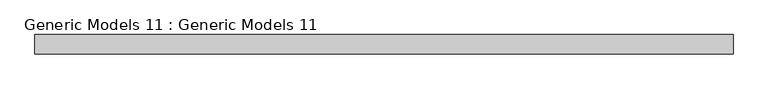
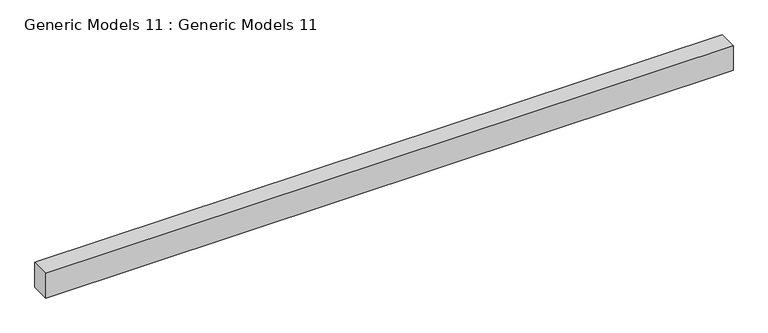
"""IFC4 building model written with IfcOpenShell, lengths in millimetres: proxy geometry, Generic Models 11 : Generic Models 11."""

from ifc_helpers import new_model, si_unit, frame, origin, place, context, project, spatial, polyline, outline, extrude, source, transform, mapped, element, save


def generic_models_11_generic_models_11_cbfe9a59(model_context):
    return source(origin(), model_context, "Body", "SweptSolid", [
        extrude(outline(polyline([(3293.0540347, -21150.5985361), (-7701.088074, -21150.5985361), (-7701.088074, -20845.7985361), (3293.0540347, -20845.7985361), (3293.0540347, -21150.5985361)])), frame((0.0, 0.0, 5983.8647714), z_axis=(0.0, 0.0, 1.0), x_axis=(1.0, 0.0, 0.0)), (0.0, 0.0, 1.0), 416.9352286),
    ])


if __name__ == "__main__":
    model = new_model("IFC4")
    model_context = context("Model", 3, world=origin())
    ifc_project = project(units=[si_unit("LENGTHUNIT", "METRE", prefix="MILLI")], contexts=[model_context])
    site = spatial("IfcSite", under=ifc_project)
    building = spatial("IfcBuilding", under=site)
    placement = place(None, origin())
    generic_models_11_generic_models_11_shape = generic_models_11_generic_models_11_cbfe9a59(model_context)
    element("IfcBuildingElementProxy", 1, Name="Generic Models 11 : Generic Models 11", ObjectType="Generic Models 11 : Generic Models 11", at=placement, inside=building, context=model_context, shape_type="MappedRepresentation", body=[
        mapped(generic_models_11_generic_models_11_shape, transform((0.0, 0.0, 0.0), x_axis=(1.0, 0.0, 0.0), y_axis=(0.0, 1.0, 0.0), z_axis=(0.0, 0.0, 1.0))),
    ])
    save(model, "model.ifc")
